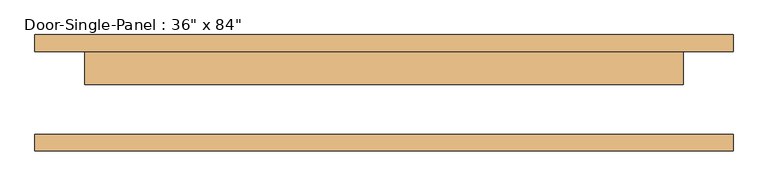
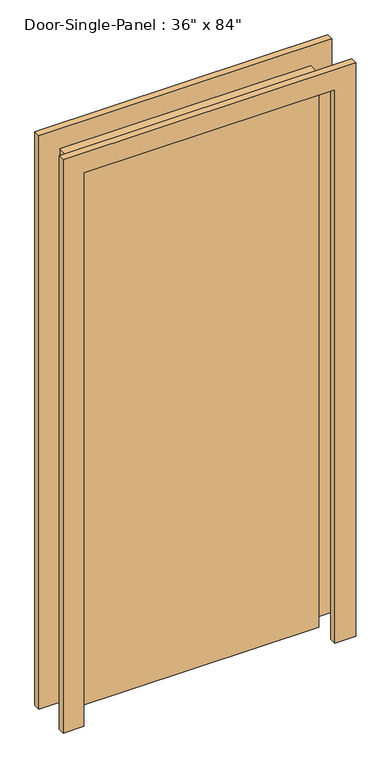
"""IFC4 building model written with IfcOpenShell, lengths in millimetres: door geometry."""

from ifc_helpers import new_model, si_unit, frame, origin, origin_with_axes, place, context, project, spatial, polyline, outline, extrude, source, transform, mapped, element, save


def door_0715e8d2(model_context):
    return source(origin(), model_context, "Body", "SweptSolid", [
        extrude(outline(polyline([(457.2, 12.7), (-457.2, 12.7), (-457.2, 63.5), (457.2, 63.5), (457.2, 12.7)])), origin_with_axes(), (0.0, 0.0, 1.0), 2133.6),
        extrude(outline(polyline([(2209.8, 533.4), (2209.8, -533.4), (0.0, -533.4), (0.0, -457.2), (2133.6, -457.2), (2133.6, 457.2), (0.0, 457.2), (0.0, 533.4), (2209.8, 533.4)])), frame((0.0, -88.9, 0.0), z_axis=(0.0, 1.0, 0.0), x_axis=(0.0, 0.0, 1.0)), (0.0, 0.0, 1.0), 25.4),
        extrude(outline(polyline([(2209.8, -533.4), (0.0, -533.4), (0.0, -457.2), (2133.6, -457.2), (2133.6, 457.2), (0.0, 457.2), (0.0, 533.4), (2209.8, 533.4), (2209.8, -533.4)])), frame((0.0, 63.5, 0.0), z_axis=(0.0, 1.0, 0.0), x_axis=(0.0, 0.0, 1.0)), (0.0, 0.0, 1.0), 25.4),
    ])


if __name__ == "__main__":
    model = new_model("IFC4")
    model_context = context("Model", 3, world=origin())
    ifc_project = project(units=[si_unit("LENGTHUNIT", "METRE", prefix="MILLI")], contexts=[model_context])
    site = spatial("IfcSite", under=ifc_project)
    building = spatial("IfcBuilding", under=site)
    placement = place(None, origin())
    door_shape = door_0715e8d2(model_context)
    element("IfcDoor", 1, ObjectType="Door-Single-Panel : 36\" x 84\"", at=placement, inside=building, context=model_context, shape_type="MappedRepresentation", body=[
        mapped(door_shape, transform((0.0, 0.0, 0.0), x_axis=(1.0, 0.0, 0.0), y_axis=(0.0, 1.0, 0.0), z_axis=(0.0, 0.0, 1.0))),
    ])
    save(model, "model.ifc")

# Revit data of these elements
# Type "Door-Single-Panel : 36\" x 84\""
#   Type Mark = "8"
#   Construction Type Id = "DOOR"
#   Assembly Code = "C1020300"
#   Analytic Construction = "Wooden"
#   Thickness = 0' - 2"
#   Thermal Resistance (R) = 2.5876 (h·ft²·°F)/BTU
#   Swing Angle [instance default] = 90.00°
#   Heat Transfer Coefficient (U) = 0.3865 BTU/(h·ft²·°F)
#   Height = 7' - 0"
#   Trim Projection Ext = 0' - 1"
#   Trim Projection Int = 0' - 1"
#   Trim Width = 0' - 3"
#   Width = 3' - 0"
#   Define Thermal Properties by = 1
#   Panel Material = Wood - Birch - Solid Stained Light Low Gloss
#   Trim Material = Paint - Sienna
#   Visual Light Transmittance = 0
#   Solar Heat Gain Coefficient = 0
#   Function = (empty or 0)
#   Wall Closure = (empty or 0)
# Element 1 (IfcDoor, "Door-Single-Panel : 36\" x 84\"")
#   Materials on its faces: "Paint - Sienna", "Wood - Birch - Solid Stained Light Low Gloss"
# Materials
#   "Wood - Birch - Solid Stained Light Low Gloss": class "Wood", colour RGB 210 159 95, transparency 0, Cost = 0
#   "Paint - Sienna": colour RGB 118 70 51, transparency 0, Cost = 0
